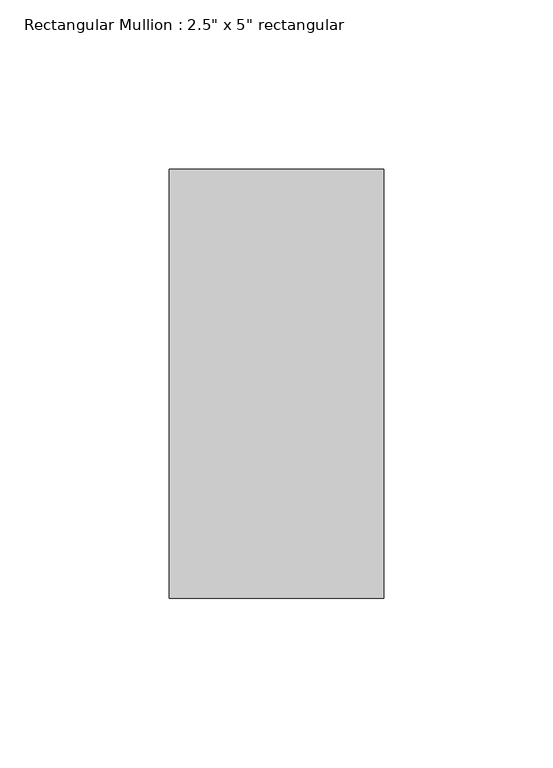
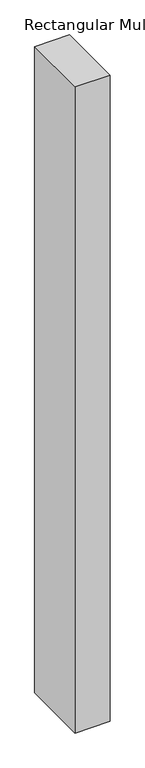
"""IFC4 building model written with IfcOpenShell, lengths in millimetres: member geometry."""

from ifc_helpers import new_model, si_unit, frame, origin, place, context, project, spatial, polyline, outline, extrude, source, transform, mapped, element, save


def member_118fc41a(model_context):
    return source(origin(), model_context, "Body", "SweptSolid", [
        extrude(outline(polyline([(0.0, 63.5), (0.0, -63.5), (-63.5, -63.5), (-63.5, 63.5), (0.0, 63.5)])), frame((0.0, 0.0, -1239.1384032), z_axis=(0.0, 0.0, 1.0), x_axis=(1.0, 0.0, 0.0)), (0.0, 0.0, 1.0), 1239.1384032),
    ])


if __name__ == "__main__":
    model = new_model("IFC4")
    model_context = context("Model", 3, world=origin())
    ifc_project = project(units=[si_unit("LENGTHUNIT", "METRE", prefix="MILLI")], contexts=[model_context])
    site = spatial("IfcSite", under=ifc_project)
    building = spatial("IfcBuilding", under=site)
    placement = place(None, origin())
    member_shape = member_118fc41a(model_context)
    element("IfcMember", 1, ObjectType="Rectangular Mullion : 2.5\" x 5\" rectangular", at=placement, inside=building, context=model_context, shape_type="MappedRepresentation", body=[
        mapped(member_shape, transform((0.0, 0.0, 0.0), x_axis=(1.0, 0.0, 0.0), y_axis=(0.0, 1.0, 0.0), z_axis=(0.0, 0.0, 1.0))),
    ])
    save(model, "model.ifc")

# Revit data of these elements
# Type "Rectangular Mullion : 2.5\" x 5\" rectangular"
#   built-in parameter 1007304 = 0.416667 (stored number, unit not read)
#   built-in parameter 1007301 = 0.104167 (stored number, unit not read)
#   built-in parameter 1007300 = 0.104167 (stored number, unit not read)
# Element 1 (IfcMember, "Rectangular Mullion : 2.5\" x 5\" rectangular")
#   Materials on its faces: "Aluminum"
# Materials
#   "Aluminum": class "Metal", colour RGB 247 247 247, transparency 0, Description = "Aluminum 6061", Cost = 0
